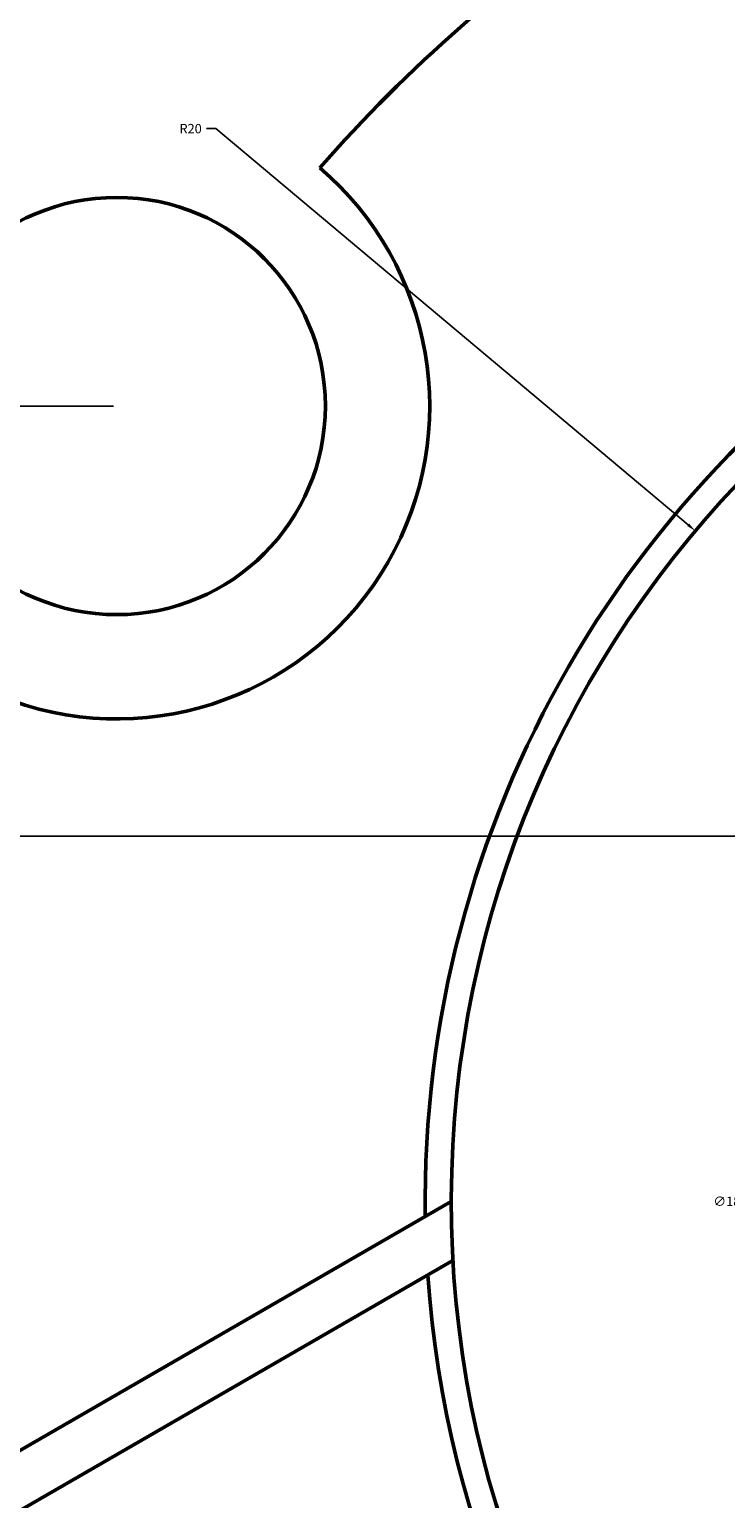
# Model space of a CAD drawing. Units: inches. Extents: x -19.9 to 72.3, y -39.8 to 57.5.
# Tile 4 of 8: x 0 to 13.3, y 7.6 to 35.8. Entities that reach past the tile are written whole.
import ezdxf

# ---------------------------------------------------------------- set-up
doc = ezdxf.new("R2010")
doc.units = ezdxf.units.IN
doc.header["$MEASUREMENT"] = 0
for name, color, linetype, lineweight in [('M-DIMS', 2, 'Continuous', 18), ('M-OUTL', 7, 'Continuous', 50), ('M-OUTL-HOLE', 7, 'Continuous', 50), ('M-OUTL-SLOT', 7, 'Continuous', 50)]:
    doc.layers.add(name, color=color, linetype=linetype, lineweight=lineweight)
doc.styles.get("Standard").update_dxf_attribs({"font": 'arial.ttf'})
doc.dimstyles.get("Standard").update_dxf_attribs({"dimtxt": 0.18, "dimasz": 0.18, "dimexe": 0.18, "dimexo": 0.0625, "dimgap": 0.09, "dimtad": 0, "dimtih": 1, "dimtoh": 1, "dimdec": 4, "dimzin": 0, "dimdsep": 46, "dimtxsty": 'Standard', "dimcen": 0.09, "dimadec": 0, "dimazin": 0, "dimtfac": 1, "dimtdec": 4, "dimtofl": 0, "dimtmove": 0, "dimatfit": 3, "dimfxl": 1, "dimtolj": 1, "dimtzin": 0, "dimarcsym": 0})

# ---------------------------------------------------------------- blocks, each defined once
blk = doc.blocks.new('FLANGE-MOUNT-D8-RELIEVED')
blk.add_circle((0, 0), 4)
for centre, radius, start, end in [((26.414, -15.25), 30, 109.4712, 138.6562), ((0, 0), 6, 250.4286, 49.5714)]:
    blk.add_arc(centre, radius, start, end)
blk = doc.blocks.new('FLANGE-STRAIGHT-SLOT')
for p, q in [((0, 0), (0, 21.114)), ((1, -0.54), (1, 20.869))]:
    blk.add_line(p, q)
blk = doc.blocks.new('*D9')
at = {"layer": 'Defpoints', "color": 0, "transparency": 16777216}
for p in [(15.936, 20.341), (-15.966, -0.659), (28.06, -0.659)]:
    blk.add_point(p, dxfattribs=at)
at = {"layer": 'M-DIMS', "color": 0, "lineweight": -2, "transparency": 16777216}
for p, q in [((15.873, 20.341), (-16.146, 20.341)), ((-15.966, 20.161), (-15.966, 10.022)), ((-15.966, -0.479), (-15.966, 9.661)), ((27.997, -0.659), (-16.146, -0.659))]:
    blk.add_line(p, q, dxfattribs=at)
at = {"layer": 'M-DIMS', "color": 0, "transparency": 16777216}
for points in [[(-15.996, 20.161), (-15.936, 20.161), (-15.966, 20.341)], [(-15.996, -0.479), (-15.936, -0.479), (-15.966, -0.659)]]:
    blk.add_solid(points, dxfattribs=at)
at = {"layer": 'M-DIMS', "color": 0, "transparency": 16777216, "insert": (-15.966, 9.841), "char_height": 0.18, "attachment_point": 5}
blk.add_mtext('\\A1;21', dxfattribs=at)
blk = doc.blocks.new('*D10')
at = {"layer": 'Defpoints', "color": 0, "transparency": 16777216}
for p in [(28.06, 43.841), (-15.966, 28.591), (1.646, 28.591)]:
    blk.add_point(p, dxfattribs=at)
at = {"layer": 'M-DIMS', "color": 0, "lineweight": -2, "transparency": 16777216}
for p, q in [((27.997, 43.841), (-16.146, 43.841)), ((-15.966, 43.661), (-15.966, 36.398)), ((-15.966, 28.771), (-15.966, 36.034)), ((1.584, 28.591), (-16.146, 28.591))]:
    blk.add_line(p, q, dxfattribs=at)
at = {"layer": 'M-DIMS', "color": 0, "transparency": 16777216}
for points in [[(-15.996, 43.661), (-15.936, 43.661), (-15.966, 43.841)], [(-15.996, 28.771), (-15.936, 28.771), (-15.966, 28.591)]]:
    blk.add_solid(points, dxfattribs=at)
at = {"layer": 'M-DIMS', "color": 0, "transparency": 16777216, "insert": (-15.966, 36.216), "char_height": 0.18, "attachment_point": 5}
blk.add_mtext('\\A1;15.25', dxfattribs=at)
blk = doc.blocks.new('*D11')
at = {"layer": 'Defpoints', "color": 0, "transparency": 16777216}
for p in [(5.703, 46.51), (50.417, -19.828)]:
    blk.add_point(p, dxfattribs=at)
at = {"layer": 'M-DIMS', "color": 0, "lineweight": -2, "transparency": 16777216}
for p, q in [((27.97, 13.341), (28.15, 13.341)), ((28.06, 13.251), (28.06, 13.431)), ((63.831, -39.729), (50.517, -19.977)), ((64.011, -39.729), (63.831, -39.729))]:
    blk.add_line(p, q, dxfattribs=at)
at = {"layer": 'M-DIMS', "color": 0, "transparency": 16777216}
blk.add_solid([(50.542, -19.96), (50.492, -19.994), (50.417, -19.828)], dxfattribs=at)
at = {"layer": 'M-DIMS', "color": 0, "transparency": 16777216, "insert": (64.327, -39.729), "char_height": 0.18, "attachment_point": 5}
blk.add_mtext('\\A1;∅80', dxfattribs=at)
blk = doc.blocks.new('*D12')
at = {"layer": 'Defpoints', "color": 0, "transparency": 16777216}
for p in [(28.06, 13.341), (-1.285, 3.349)]:
    blk.add_point(p, dxfattribs=at)
at = {"layer": 'M-DIMS', "color": 0, "lineweight": -2, "transparency": 16777216}
for p, q in [((27.97, 13.341), (28.15, 13.341)), ((28.06, 13.251), (28.06, 13.431)), ((-18.893, -2.647), (-1.456, 3.291)), ((-19.073, -2.647), (-18.893, -2.647))]:
    blk.add_line(p, q, dxfattribs=at)
at = {"layer": 'M-DIMS', "color": 0, "transparency": 16777216}
blk.add_solid([(-1.466, 3.319), (-1.446, 3.262), (-1.285, 3.349)], dxfattribs=at)
at = {"layer": 'M-DIMS', "color": 0, "transparency": 16777216, "insert": (-19.557, -2.647), "char_height": 0.18, "attachment_point": 5}
blk.add_mtext('\\A1;4X R31', dxfattribs=at)
blk = doc.blocks.new('*D13')
at = {"layer": 'Defpoints', "color": 0, "transparency": 16777216}
for p in [(11.256, 38.194), (28.06, 13.341)]:
    blk.add_point(p, dxfattribs=at)
at = {"layer": 'M-DIMS', "color": 0, "lineweight": -2, "transparency": 16777216}
for p, q in [((0.994, 53.105), (1.174, 53.105)), ((1.174, 53.105), (11.155, 38.343)), ((27.97, 13.341), (28.15, 13.341)), ((28.06, 13.251), (28.06, 13.431))]:
    blk.add_line(p, q, dxfattribs=at)
at = {"layer": 'M-DIMS', "color": 0, "transparency": 16777216}
blk.add_solid([(11.18, 38.36), (11.131, 38.326), (11.256, 38.194)], dxfattribs=at)
at = {"layer": 'M-DIMS', "color": 0, "transparency": 16777216, "insert": (0.434, 53.105), "char_height": 0.18, "attachment_point": 5}
blk.add_mtext('\\A1;10X R30', dxfattribs=at)
blk = doc.blocks.new('*D15')
at = {"layer": 'Defpoints', "color": 0, "transparency": 16777216}
for p in [(12.739, 26.197), (28.06, 13.341)]:
    blk.add_point(p, dxfattribs=at)
at = {"layer": 'M-DIMS', "color": 0, "lineweight": -2, "transparency": 16777216}
for p, q in [((3.366, 33.91), (3.546, 33.91)), ((3.546, 33.91), (12.601, 26.313)), ((27.97, 13.341), (28.15, 13.341)), ((28.06, 13.251), (28.06, 13.431))]:
    blk.add_line(p, q, dxfattribs=at)
at = {"layer": 'M-DIMS', "color": 0, "transparency": 16777216}
blk.add_solid([(12.62, 26.336), (12.582, 26.29), (12.739, 26.197)], dxfattribs=at)
at = {"layer": 'M-DIMS', "color": 0, "transparency": 16777216, "insert": (3.062, 33.91), "char_height": 0.18, "attachment_point": 5}
blk.add_mtext('\\A1;R20', dxfattribs=at)
blk = doc.blocks.new('*D19')
at = {"layer": 'Defpoints', "color": 0, "transparency": 16777216}
for p in [(19.06, 13.341), (37.06, 13.342)]:
    blk.add_point(p, dxfattribs=at)
at = {"layer": 'M-DIMS', "color": 0, "lineweight": -2, "transparency": 16777216}
for p, q in [((13.66, 13.341), (18.88, 13.341)), ((27.97, 13.341), (28.15, 13.341)), ((28.06, 13.251), (28.06, 13.431))]:
    blk.add_line(p, q, dxfattribs=at)
at = {"layer": 'M-DIMS', "color": 0, "transparency": 16777216}
blk.add_solid([(18.88, 13.371), (18.88, 13.311), (19.06, 13.341)], dxfattribs=at)
at = {"layer": 'M-DIMS', "color": 0, "transparency": 16777216, "insert": (13.343, 13.341), "char_height": 0.18, "attachment_point": 5}
blk.add_mtext('\\A1;∅18', dxfattribs=at)

msp = doc.modelspace()

# ---------------------------------------------------------------- linework, layer by layer
at = {"layer": 'M-OUTL'}
msp.add_circle((28.06, 13.341), 40, dxfattribs=at)
for radius, start, end in [(20, 0, 356.7437), (20.5, 119.1964, 180.8036), (20.5, 183.9584, 60.8036)]:
    msp.add_arc((28.06, 13.341), radius, start, end, dxfattribs=at)

# ---------------------------------------------------------------- block references
at = {"layer": 'M-OUTL-HOLE'}
msp.add_blockref('FLANGE-MOUNT-D8-RELIEVED', (1.646, 28.591), dxfattribs=at)
at = {"layer": 'M-OUTL-SLOT', "rotation": 119.9999999999999}
msp.add_blockref('FLANGE-STRAIGHT-SLOT', (8.092, 12.205), dxfattribs=at)

# ---------------------------------------------------------------- dimensions: what is measured, and where the dimension line sits
at = {"layer": 'M-DIMS'}
for mpoint, text, picture, middle in [((11.256, 38.194), '10X <>', '*D13', (0.434, 53.105)), ((-1.285, 3.349), '4X <>', '*D12', (-19.557, -2.647))]:
    dim = msp.add_radius_dim(center=(28.06, 13.341), mpoint=mpoint, text=text, dimstyle='Standard', override={"dimdec": 0, "dimlfac": 1, "dimrnd": 0, "dimzin": 0, "dimdsep": 46, "dimlunit": 2}, dxfattribs=at)
    dim.commit()
    dim.dimension.update_dxf_attribs({"geometry": picture, "text_midpoint": middle, "dimtype": 164})
for p1, p2, picture, middle in [((5.703, 46.51), (50.417, -19.828), '*D11', (64.327, -39.729)), ((37.06, 13.342), (19.06, 13.341), '*D19', (13.66, 13.341))]:
    dim = msp.add_diameter_dim_2p(p1=p1, p2=p2, dimstyle='Standard', override={"dimdec": 0, "dimlfac": 1, "dimrnd": 0, "dimzin": 0, "dimdsep": 46, "dimlunit": 2}, dxfattribs=at)
    dim.commit()
    dim.dimension.update_dxf_attribs({"geometry": picture, "text_midpoint": middle, "dimtype": 163})
for base, p1, p2, override, picture, middle in [((-15.966, 28.591), (28.06, 43.841), (1.646, 28.591), {"dimdec": 2, "dimlfac": 1, "dimrnd": 0, "dimzin": 0, "dimdsep": 46, "dimlunit": 2}, '*D10', (-15.966, 36.216)), ((-15.966, -0.659), (15.936, 20.341), (28.06, -0.659), {"dimdec": 0, "dimlfac": 1, "dimrnd": 0, "dimzin": 0, "dimdsep": 46, "dimlunit": 2}, '*D9', (-15.966, 9.841))]:
    dim = msp.add_linear_dim(base=base, p1=p1, p2=p2, angle=90, dimstyle='Standard', override=override, dxfattribs=at)
    dim.commit()
    dim.dimension.update_dxf_attribs({"geometry": picture, "text_midpoint": middle})
dim = msp.add_radius_dim(center=(28.06, 13.341), mpoint=(12.739, 26.197), dimstyle='Standard', override={"dimdec": 0, "dimlfac": 1, "dimrnd": 0, "dimzin": 0, "dimdsep": 46, "dimlunit": 2}, dxfattribs=at)
dim.commit()
dim.dimension.update_dxf_attribs({"geometry": '*D15', "text_midpoint": (3.062, 33.91), "dimtype": 164})

doc.saveas('drawing.dxf')
